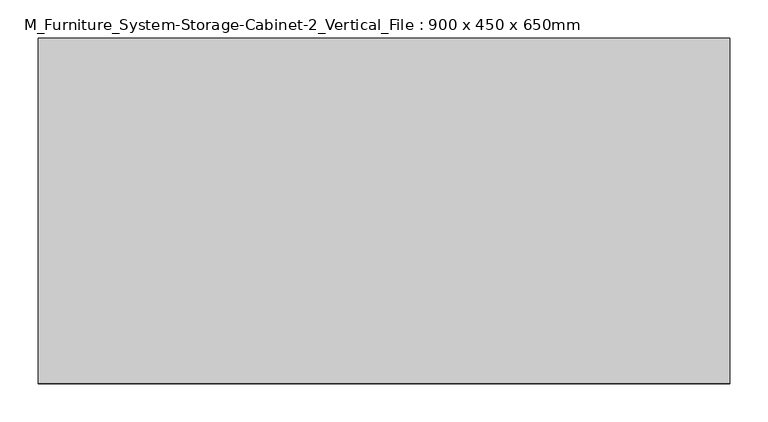
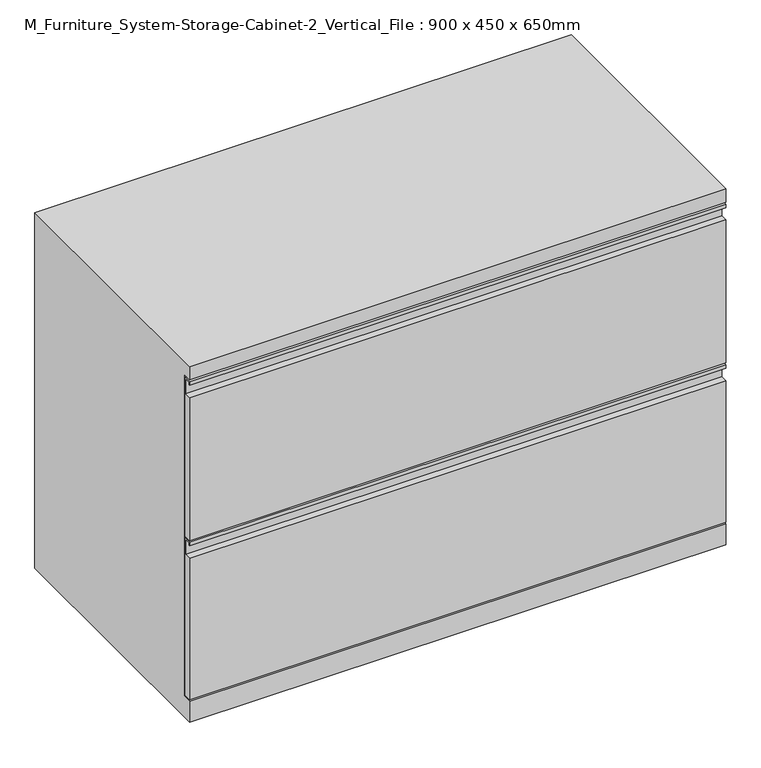
"""IFC4 building model written with IfcOpenShell, lengths in millimetres: furniture geometry, M_Furniture_System-Storage-Cabinet-2_Vertical_File : 900 x 450 x 650mm."""

from ifc_helpers import new_model, si_unit, frame, origin, place, context, project, spatial, polyline, outline, extrude, source, transform, mapped, element, save


def m_furniture_system_storage_cabinet_2_vertical_file_900_x_450_def3fd80(model_context):
    return source(origin(), model_context, "Body", "SweptSolid", [
        extrude(outline(polyline([(0.0, 341.2718803), (0.0, 594.8451302), (11.8998876, 594.8451302), (11.8998876, 621.4884893), (1.5239879, 621.4884893), (1.5239879, 616.6625121), (0.0, 616.6625121), (0.0, 623.0124879), (13.4873883, 623.0124879), (13.4873883, 341.2718803), (0.0, 341.2718803)])), frame((-450.0, 0.0, 0.0), z_axis=(1.0, 0.0, 0.0), x_axis=(0.0, 1.0, 0.0)), (0.0, 0.0, 1.0), 900.0),
        extrude(outline(polyline([(0.0, 58.7374985), (0.0, 309.9295347), (11.9293774, 309.9295347), (11.9293774, 336.5728939), (1.5239879, 336.5728939), (1.5239879, 331.7468803), (0.0, 331.7468803), (0.0, 338.0968924), (13.4873883, 338.0968924), (13.4873883, 58.7374985), (0.0, 58.7374985)])), frame((-450.0, 0.0, 0.0), z_axis=(1.0, 0.0, 0.0), x_axis=(0.0, 1.0, 0.0)), (0.0, 0.0, 1.0), 900.0),
        extrude(outline(polyline([(56.820048, 9.2063177), (51.9174039, 19.05), (100.4825718, 19.05), (95.5799278, 9.2063177), (86.9277397, 2.4185626), (76.1999879, 0.0), (65.4722406, 2.4185626), (56.820048, 9.2063177)])), frame((-396.025, 0.0, 0.0), z_axis=(1.0, 0.0, 0.0), x_axis=(0.0, 1.0, 0.0)), (0.0, 0.0, 1.0), 44.45),
        extrude(outline(polyline([(354.4200601, 9.2063177), (349.517416, 19.05), (398.082584, 19.05), (393.1799399, 9.2063177), (384.5277518, 2.4185626), (373.8, 0.0), (363.0722527, 2.4185626), (354.4200601, 9.2063177)])), frame((-396.025, 0.0, 0.0), z_axis=(1.0, 0.0, 0.0), x_axis=(0.0, 1.0, 0.0)), (0.0, 0.0, 1.0), 44.45),
        extrude(outline(polyline([(56.820048, 9.2063177), (51.9174039, 19.05), (100.4825718, 19.05), (95.5799278, 9.2063177), (86.9277397, 2.4185626), (76.1999879, 0.0), (65.4722406, 2.4185626), (56.820048, 9.2063177)])), frame((351.575, 0.0, 0.0), z_axis=(1.0, 0.0, 0.0), x_axis=(0.0, 1.0, 0.0)), (0.0, 0.0, 1.0), 44.45),
        extrude(outline(polyline([(398.082584, 19.05), (393.1799399, 9.2063177), (384.5277518, 2.4185626), (373.8, 0.0), (363.0722527, 2.4185626), (354.4200601, 9.2063177), (349.517416, 19.05), (398.082584, 19.05)])), frame((351.575, 0.0, 0.0), z_axis=(1.0, 0.0, 0.0), x_axis=(0.0, 1.0, 0.0)), (0.0, 0.0, 1.0), 44.45),
        extrude(outline(polyline([(0.0, 650.0), (450.0, 650.0), (450.0, 19.05), (0.0, 19.05), (0.0, 56.3562485), (16.6623883, 56.3562485), (16.6623883, 626.1875121), (0.0, 626.1875121), (0.0, 650.0)])), frame((-450.0, 0.0, 0.0), z_axis=(1.0, 0.0, 0.0), x_axis=(0.0, 1.0, 0.0)), (0.0, 0.0, 1.0), 900.0),
    ])


if __name__ == "__main__":
    model = new_model("IFC4")
    model_context = context("Model", 3, world=origin())
    ifc_project = project(units=[si_unit("LENGTHUNIT", "METRE", prefix="MILLI")], contexts=[model_context])
    site = spatial("IfcSite", under=ifc_project)
    building = spatial("IfcBuilding", under=site)
    placement = place(None, origin())
    m_furniture_system_storage_cabinet_2_vertical_file_900_x_450_shape = m_furniture_system_storage_cabinet_2_vertical_file_900_x_450_def3fd80(model_context)
    element("IfcFurniture", 1, ObjectType="M_Furniture_System-Storage-Cabinet-2_Vertical_File : 900 x 450 x 650mm", at=placement, inside=building, context=model_context, shape_type="MappedRepresentation", body=[
        mapped(m_furniture_system_storage_cabinet_2_vertical_file_900_x_450_shape, transform((0.0, 0.0, 0.0), x_axis=(1.0, 0.0, 0.0), y_axis=(0.0, 1.0, 0.0), z_axis=(0.0, 0.0, 1.0))),
    ])
    save(model, "model.ifc")

# Revit data of these elements
# Type "M_Furniture_System-Storage-Cabinet-2_Vertical_File : 900 x 450 x 650mm"
#   Type Comments = "900 x 450 x 650mm Double Vertical File Cabinet"
#   Width = 2.952756 ft
#   Height = 2.132546 ft
#   Depth = 1.476378 ft
#   Show Solid [instance default] = yes
#   Show Dashed [instance default] = no
#   Drawer Finish [instance default] = Metal - Paint - Beige
#   Cabinet Material [instance default] = Metal - Paint - Beige
#   Model = ""
#   Manufacturer = ""
#   Description = (empty or 0)
#   Default Elevation = 0
# Element 1 (IfcFurniture, "M_Furniture_System-Storage-Cabinet-2_Vertical_File : 900 x 450 x 650mm")
#   Materials on its faces: "Metal - Paint - Beige"
# Materials
#   "Metal - Paint - Beige": class "Metal", colour RGB 247 225 182, transparency 0
